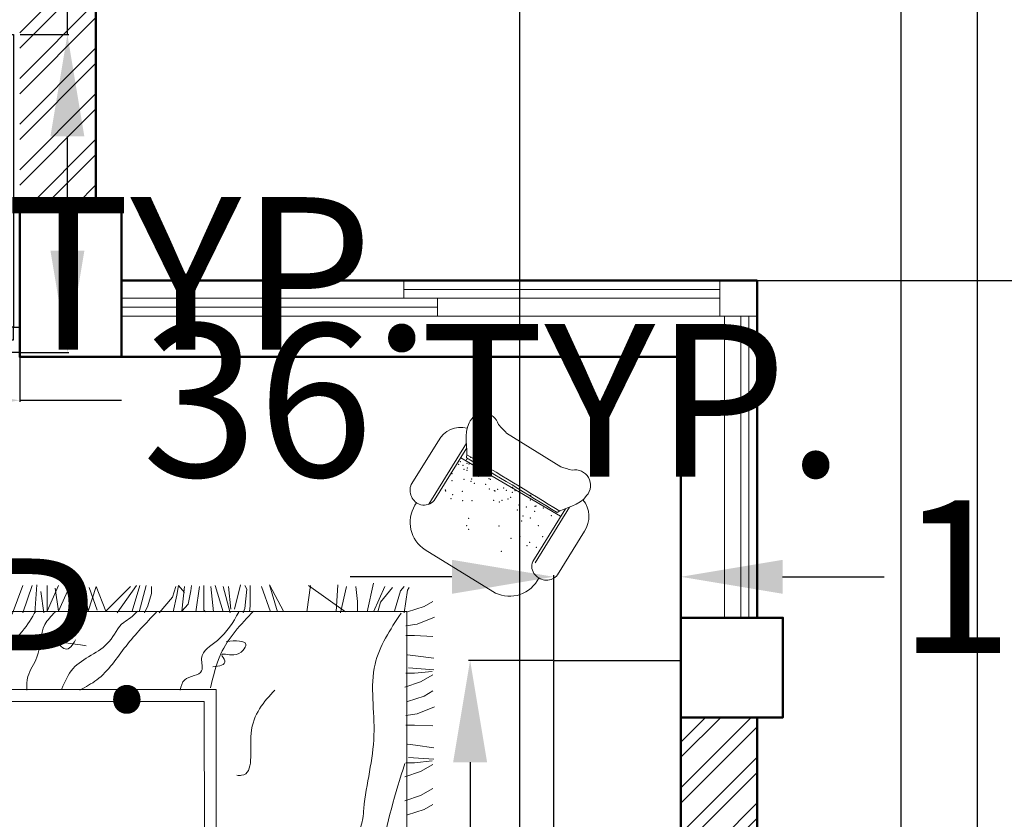
# Model space of a CAD drawing. Units: inches. Extents: x -90 to 536, y -553 to 299.
# Tile 25 of 27: x 294 to 410, y 80 to 174. Entities that reach past the tile are written whole.
import ezdxf

# ---------------------------------------------------------------- set-up
doc = ezdxf.new("R2010")
doc.units = ezdxf.units.IN
for name, color, linetype, lineweight in [('A-ANNO-DIMS', 2, 'Continuous', 18), ('A-COLS', 7, 'Continuous', 50), ('A-DOOR', 4, 'Continuous', 25), ('A-FLOR-CASE', 2, 'Continuous', 25), ('A-GLAZ', 4, 'Continuous', 18), ('A-WALL-PATT', 252, 'Continuous', 13), ('Furniture', 2, 'Continuous', 18), ('Outer Wall', 1, 'Continuous', 50)]:
    doc.layers.add(name, color=color, linetype=linetype, lineweight=lineweight)
doc.styles.get("Standard").update_dxf_attribs({"font": 'arial.ttf'})
doc.dimstyles.get("Standard").update_dxf_attribs({"dimtxt": 18, "dimasz": 12, "dimexe": 0.18, "dimexo": 0.0625, "dimgap": 0.09, "dimtad": 0, "dimtih": 1, "dimtoh": 1, "dimdec": 0, "dimzin": 0, "dimdsep": 46, "dimlunit": 3, "dimtxsty": 'Standard', "dimcen": 0.09, "dimadec": 0, "dimazin": 0, "dimtfac": 1, "dimtdec": 0, "dimtofl": 0, "dimtmove": 0, "dimatfit": 3, "dimfxl": 1, "dimtolj": 1, "dimtzin": 0, "dimarcsym": 0})

# ---------------------------------------------------------------- blocks, each defined once
blk = doc.blocks.new('A$C14440869')
for p, q in [((299.4, 786.8), (654.5, 786.8)), ((141.1, 259.3), (141.1, 621.8)), ((154.9, 258.1), (156.1, 601.9)), ((799, 258.1), (797.7, 601.9)), ((812.8, 224.7), (812.8, 621.8)), ((0, 267.1), (1, 551.8)), ((798, 537.4), (157.2, 552.6)), ((953.9, 267.1), (952.8, 551.8)), ((78.7, 198), (78.7, 179.8)), ((875.1, 196.3), (875.2, 179.8)), ((257.3, 0.1), (696.7, 0))]:
    blk.add_line(p, q)
for centre, radius, start, end in [((178, 741.7), 84.9, 46.4058, 190.9946), ((775.9, 741.7), 84.9, 349.0054, 133.5942), ((490.5, 1647.2), 881.3, 253.2515, 257.4746), ((463.3, 1647.2), 881.3, 282.5254, 286.7485), ((146, 557.8), 145.1, 108.7163, 182.3743), ((810.8, 559.8), 142.3, 356.766, 72.1434), ((234.9, -29958.2), 30532.1, 88.98134, 90.11086), ((164.3, -28909.7), 29469.6, 88.82111, 89.96326), ((79.9, 278.7), 80.7, 188.2473, 288.8842), ((90.3, 265.5), 65, 283.9696, 353.4821), ((871.6, 268.6), 73.4, 188.2144, 251.9677), ((869.8, 281.5), 85.3, 255.8372, 350.3327), ((257.8, 179.2), 179.2, 179.795, 269.795), ((696, 179.2), 179.2, 270.205, 0.205)]:
    blk.add_arc(centre, radius, start, end)
for points in [[(94.6, 725.5), (94.6, 660.2), (167.2, 599.5), (183.2, 559.8)], [(859.3, 725.5), (859.3, 660.2), (786.7, 599.5), (770.6, 553.6)]]:
    blk.add_open_spline(points, degree=3)
for p in [(358.4, 564.7), (467, 548.6), (656.1, 560.7), (752.6, 568.7), (201.4, 528.5), (261.8, 540.6), (294, 500.4), (302, 528.5), (306.1, 524.5), (346.3, 540.6), (346.3, 496.4), (446.9, 540.6), (446.9, 496.4), (454.9, 524.5), (487.1, 516.5), (507.2, 520.5), (531.4, 496.4), (595.7, 520.5), (603.8, 520.5), (647.8, 524.5), (651.8, 528.5), (656.1, 532.5), (656.1, 524.5), (659.9, 500.4), (688.3, 492.3), (692.1, 540.6), (696.3, 520.5), (700.3, 528.5), (732.5, 496.4), (736.6, 508.4), (740.6, 532.5), (748.6, 492.3), (752.4, 528.5), (764.7, 544.6), (764.7, 508.4), (788.9, 516.5), (788.9, 500.4), (233.6, 444.1), (294, 456.2), (334.2, 444.1), (378.5, 456.2), (386.5, 484.3), (454.9, 480.3), (479.1, 456.2), (487.1, 440.1), (539.4, 480.3), (543.4, 480.3), (571.6, 472.3), (603.8, 484.3), (659.9, 456.2), (680.2, 456.2), (684.2, 468.2), (720.2, 444.1), (181.3, 403.9), (326.2, 416), (519.3, 432.1), (692.3, 383.9), (772.5, 403.9), (792.9, 436.1), (181.3, 335.6), (225.6, 339.6), (290, 339.6), (418.7, 327.6), (619.9, 367.8), (663.9, 339.6), (728.3, 339.6), (772.5, 335.6), (776.8, 339.6), (229.6, 315.5), (326.2, 303.5), (583.7, 275.4), (724.3, 315.5), (551.5, 223.1), (571.6, 235.2), (334.2, 215.1)]:
    blk.add_point(p)
blk = doc.blocks.new('A$C2B723114')
for p, q in [((2.1776, 2.8509), (2.1776, 0.7454)), ((2.216, 2.8509), (2.216, 0.707)), ((2.4685, 1.4964), (2.4685, 0.0903)), ((2.4596, 1.3659), (2.552, 1.3324)), ((2.4645, 1.3318), (2.552, 1.3012)), ((2.4645, 1.2928), (2.5548, 1.2871)), ((2.4645, 1.2635), (2.5328, 1.2733)), ((2.4699, 1.2531), (2.552, 1.2163)), ((2.552, 1.2531), (2.4699, 1.2531)), ((2.5435, 1.2276), (2.4699, 1.2163)), ((2.4699, 1.2163), (2.5463, 1.1823)), ((2.5491, 1.1654), (2.467, 1.1597)), ((2.5463, 1.1455), (2.467, 1.1342)), ((2.5491, 1.1342), (2.4699, 1.1201)), ((2.4699, 1.1201), (2.5491, 1.0946)), ((2.5463, 1.1172), (2.4727, 1.0918)), ((2.5491, 1.0946), (2.4699, 1.0635)), ((2.4699, 1.0635), (2.5491, 0.9842)), ((2.4642, 1.0267), (2.552, 0.9644)), ((2.467, 0.9559), (2.552, 0.9333)), ((2.4699, 0.9785), (2.552, 0.9531)), ((2.4642, 0.9389), (2.4869, 0.9276)), ((2.4869, 0.9276), (2.5265, 0.9163)), ((2.5265, 0.9163), (2.5491, 0.9163)), ((2.4642, 0.8908), (2.5152, 0.8483)), ((2.467, 0.8455), (2.5208, 0.8342)), ((2.5152, 0.8483), (2.5491, 0.837)), ((2.5208, 0.8342), (2.552, 0.8285)), ((2.552, 0.8285), (2.5293, 0.8087)), ((2.4699, 0.8172), (2.4925, 0.7974)), ((2.5491, 0.8087), (2.4699, 0.8172)), ((2.4925, 0.7974), (2.535, 0.7889)), ((2.5491, 0.7606), (2.467, 0.7719)), ((2.535, 0.7889), (2.552, 0.7861)), ((2.1776, 0.7454), (0.7187, 0.7435)), ((2.4727, 0.7464), (2.467, 0.7408)), ((2.552, 0.7464), (2.4727, 0.7464)), ((2.216, 0.707), (0.6794, 0.7051)), ((2.467, 0.7153), (2.5491, 0.7238)), ((2.552, 0.7096), (2.467, 0.6842)), ((2.5491, 0.6842), (2.4642, 0.6615)), ((2.5491, 0.6672), (2.4755, 0.6587)), ((2.4755, 0.6474), (2.5548, 0.6276)), ((2.4642, 0.6191), (2.4784, 0.6134)), ((2.4784, 0.6134), (2.5406, 0.6077)), ((2.5406, 0.6077), (2.552, 0.6134)), ((2.467, 0.5993), (2.4869, 0.5964)), ((2.4869, 0.5964), (2.552, 0.5964)), ((2.467, 0.5313), (2.5491, 0.5596)), ((2.467, 0.5087), (2.5548, 0.5342)), ((2.5548, 0.5342), (2.4699, 0.4889)), ((2.467, 0.4133), (2.552, 0.4019)), ((2.467, 0.2879), (2.552, 0.4076)), ((2.467, 0.319), (2.5548, 0.3134)), ((2.4642, 0.3049), (2.5491, 0.2851)), ((2.4699, 0.2491), (2.501, 0.2491)), ((2.501, 0.2491), (2.5491, 0.2547)), ((2.467, 0.2179), (2.5605, 0.1981)), ((2.467, 0.1981), (2.5491, 0.1613)), ((2.467, 0.184), (2.4982, 0.1755)), ((2.4982, 0.1755), (2.5463, 0.1359)), ((2.4699, 0.1302), (2.535, 0.1104)), ((1.8568, 0.0962), (1.8738, 0.0453)), ((1.9342, 0.0962), (1.9512, 0.0453)), ((2.2236, 0.0962), (2.2406, 0.0453)), ((2.4642, 0.0991), (2.5378, 0.0877)), ((2.535, 0.1104), (2.5491, 0.0991)), ((2.4685, 0.0903), (0.4269, 0.0884)), ((1.8108, 0.0877), (1.8278, 0.034)), ((1.9795, 0.0934), (1.9795, 0.0651)), ((1.9795, 0.0651), (1.9852, 0.0085)), ((1.9965, 0.0849), (1.9908, 0.0028)), ((2.039, 0.0877), (2.0361, 0.0623)), ((2.1012, 0.0651), (2.0984, 0.0057)), ((2.1012, 0.0934), (2.1012, 0.0651)), ((2.1324, 0.0934), (2.138, 0.0566)), ((2.1777, 0.0877), (2.1946, 0.034)), ((2.2689, 0.0934), (2.2689, 0.0651)), ((2.2689, 0.0651), (2.2746, 0.0085)), ((2.2859, 0.0849), (2.2802, 0.0028)), ((2.3284, 0.0877), (2.3255, 0.0623)), ((2.3906, 0.0651), (2.3878, 0.0057)), ((2.3906, 0.0934), (2.3906, 0.0651)), ((2.4218, 0.0934), (2.4274, 0.0566)), ((2.467, 0.0877), (2.484, 0.034)), ((2.5378, 0.0877), (2.5463, 0.0821)), ((1.8278, 0.034), (1.8448, 0.0057)), ((1.8738, 0.0453), (1.8964, 0.0057)), ((1.9512, 0.0453), (1.9739, 0.0057)), ((2.0361, 0.0623), (2.0276, 0.0028)), ((2.138, 0.0566), (2.1607, 0)), ((2.1946, 0.034), (2.2116, 0.0057)), ((2.2406, 0.0453), (2.2632, 0.0057)), ((2.3255, 0.0623), (2.317, 0.0028)), ((2.4274, 0.0566), (2.4501, 0)), ((2.484, 0.034), (2.501, 0.0057))]:
    blk.add_line(p, q)
for points, knots in [([(2.2145, 1.4211), (2.233, 1.4246), (2.2636, 1.4303), (2.2761, 1.3837), (2.3429, 1.3967), (2.3949, 1.3342), (2.4474, 1.3031), (2.4698, 1.2898)], [0, 0, 0, 0, 61.886907, 102.717887, 145.699352, 284.082577, 386.765171, 386.765171, 386.765171, 386.765171]), ([(2.2145, 1.319), (2.2295, 1.319), (2.2678, 1.3192), (2.3288, 1.2705), (2.4143, 1.279), (2.4535, 1.2403), (2.4662, 1.2278)], [0, 0, 0, 0, 57.155505, 146.33427, 287.936209, 355.396728, 355.396728, 355.396728, 355.396728]), ([(2.3573, 1.127), (2.3656, 1.1759), (2.3758, 1.2352), (2.3371, 1.1853), (2.3602, 1.1713), (2.3768, 1.1612)], [0, 0, 0, 0, 107.853607, 130.728419, 189.220329, 189.220329, 189.220329, 189.220329]), ([(2.2182, 1.2059), (2.2419, 1.1958), (2.3116, 1.1659), (2.342, 1.0552), (2.4266, 1.0223), (2.4474, 0.9811), (2.462, 0.9684), (2.4698, 0.9616)], [0, 0, 0, 0, 97.73655, 287.59661, 389.176293, 423.403759, 463.679181, 463.679181, 463.679181, 463.679181]), ([(2.2145, 1.1476), (2.2246, 1.1286), (2.2575, 1.0666), (2.3612, 1.0009), (2.431, 0.9336), (2.4662, 0.8996)], [0, 0, 0, 0, 83.02987, 271.460712, 463.033803, 463.033803, 463.033803, 463.033803]), ([(2.2145, 0.823), (2.227, 0.8201), (2.261, 0.8121), (2.261, 0.7401), (2.3352, 0.7659), (2.379, 0.6836), (2.4336, 0.6521), (2.4662, 0.6334)], [0, 0, 0, 0, 46.747668, 127.438174, 179.649794, 280.561838, 429.605131, 429.605131, 429.605131, 429.605131]), ([(2.2218, 0.7246), (2.2595, 0.716), (2.3548, 0.6945), (2.4265, 0.6268), (2.4698, 0.586)], [0, 0, 0, 0, 148.665024, 375.555892, 375.555892, 375.555892, 375.555892]), ([(2.3719, 0.6737), (2.3738, 0.6431), (2.3772, 0.5878), (2.3146, 0.6382), (2.3401, 0.7015), (2.2971, 0.6649), (2.2923, 0.6965), (2.289, 0.7176)], [0, 0, 0, 0, 83.446591, 150.887818, 201.642461, 230.015204, 286.760644, 286.760644, 286.760644, 286.760644]), ([(2.2145, 0.5167), (2.1764, 0.5522), (2.1051, 0.6184), (1.9357, 0.5803), (1.9385, 0.6342), (1.9388, 0.6395)], [0, 0, 0, 0, 208.073343, 389.01094, 409.01094, 409.01094, 409.01094, 409.01094]), ([(2.4625, 0.1088), (2.4095, 0.1438), (2.2904, 0.2226), (2.0623, 0.1771), (1.9006, 0.2246), (1.7699, 0.2337), (1.6941, 0.2766), (1.5528, 0.2786), (1.4005, 0.2587), (1.2324, 0.3267), (1.059, 0.2939), (0.9218, 0.426), (0.7359, 0.3204), (0.5586, 0.2391), (0.4502, 0.3116), (0.427, 0.3272)], [0, 0, 0, 0, 239.874704, 538.942419, 850.40885, 893.390315, 1047.998294, 1176.505142, 1437.500972, 1637.333004, 1864.324391, 2089.058767, 2248.736533, 2637.953392, 2744.252142, 2744.252142, 2744.252142, 2744.252142]), ([(1.9771, 0.0962), (1.9286, 0.1117), (1.7864, 0.157), (1.5223, 0.1992), (1.2611, 0.141), (1.0527, 0.2023), (0.8859, 0.1885), (0.76, 0.3042), (0.6211, 0.292), (0.5187, 0.3203), (0.4572, 0.3456), (0.4282, 0.3575)], [0, 0, 0, 0, 198.710624, 582.73994, 1031.873213, 1206.082894, 1423.278209, 1655.952104, 1808.744089, 1945.69963, 2068.229211, 2068.229211, 2068.229211, 2068.229211])]:
    blk.add_open_spline(points, degree=3, knots=knots)
blk = doc.blocks.new('DOOR-36-A')
for points in [[(35.25, 37.5), (35.25, 3), (34.5, 3), (34.5, 37.5)], [(0, 0), (1.5, 0), (1.5, 1.5), (0.75, 1.5), (0.75, 3), (0, 3)], [(36, 0), (34.5, 0), (34.5, 1.5), (35.25, 1.5), (35.25, 3), (36, 3)]]:
    blk.add_lwpolyline(points, close=True)
blk.add_arc((37.64, 1.5), 36.14, 94.9791, 180)
blk = doc.blocks.new('COL-12X18')
blk.add_lwpolyline([(0, 18), (12, 18), (12, 0), (0, 0)], close=True)
blk = doc.blocks.new('COL-WINDOW-PIER')
blk.add_lwpolyline([(0, 11.76), (12.04, 11.76), (12.04, 0), (0, 0)], close=True)
blk = doc.blocks.new('TV-UNIT')
blk.add_lwpolyline([(15, 65.77), (15, 0), (0, 0), (0, 65.77)], close=True)
blk = doc.blocks.new('*D19')
at = {"layer": 'A-ANNO-DIMS', "color": 0, "lineweight": -2, "transparency": 16777216}
for p, q in [((299.76, 172.45), (299.76, 184.45)), ((299.76, 184.45), (311.76, 184.45)), ((294.19, 172.45), (299.94, 172.45)), ((299.76, 146.95), (299.76, 160.45)), ((294.19, 134.95), (299.94, 134.95))]:
    blk.add_line(p, q, dxfattribs=at)
at = {"layer": 'A-ANNO-DIMS', "color": 0, "transparency": 16777216}
for points in [[(297.76, 160.45), (301.76, 160.45), (299.76, 172.45)], [(297.76, 146.95), (301.76, 146.95), (299.76, 134.95)]]:
    blk.add_solid(points, dxfattribs=at)
at = {"layer": 'Defpoints', "color": 0, "transparency": 16777216}
for p in [(294.13, 172.45), (299.76, 172.45), (294.13, 134.95)]:
    blk.add_point(p, dxfattribs=at)
at = {"layer": 'A-ANNO-DIMS', "color": 0, "transparency": 16777216, "insert": (408.3, 184.45), "char_height": 18, "attachment_point": 5}
blk.add_mtext('\\A1;DOOR A 38 TYP.', dxfattribs=at)
blk = doc.blocks.new('*D20')
at = {"layer": 'A-ANNO-DIMS', "color": 0, "lineweight": -2, "transparency": 16777216}
for p, q in [((258.13, 134.88), (258.13, 129.14)), ((294.13, 134.88), (294.13, 129.14)), ((270.13, 129.32), (282.13, 129.32)), ((294.13, 129.32), (306.13, 129.32))]:
    blk.add_line(p, q, dxfattribs=at)
at = {"layer": 'A-ANNO-DIMS', "color": 0, "transparency": 16777216}
for points in [[(270.13, 131.32), (270.13, 127.32), (258.13, 129.32)], [(282.13, 131.32), (282.13, 127.32), (294.13, 129.32)]]:
    blk.add_solid(points, dxfattribs=at)
at = {"layer": 'Defpoints', "color": 0, "transparency": 16777216}
for p in [(258.13, 134.95), (294.13, 134.95), (294.13, 129.32)]:
    blk.add_point(p, dxfattribs=at)
at = {"layer": 'A-ANNO-DIMS', "color": 0, "transparency": 16777216, "insert": (350.02, 129.32), "char_height": 18, "attachment_point": 5}
blk.add_mtext('\\A1;36 TYP.', dxfattribs=at)
blk = doc.blocks.new('*D25')
at = {"layer": 'A-ANNO-DIMS', "color": 0, "lineweight": -2, "transparency": 16777216}
for p, q in [((228.95, 178.94), (228.95, 190.94)), ((228.95, 190.94), (240.95, 190.94)), ((226.49, 166.94), (229.13, 166.94)), ((226.49, 150.15), (229.13, 150.15)), ((228.95, 138.15), (228.95, 126.15))]:
    blk.add_line(p, q, dxfattribs=at)
at = {"layer": 'A-ANNO-DIMS', "color": 0, "transparency": 16777216}
for points in [[(226.95, 178.94), (230.95, 178.94), (228.95, 166.94)], [(226.95, 138.15), (230.95, 138.15), (228.95, 150.15)]]:
    blk.add_solid(points, dxfattribs=at)
at = {"layer": 'Defpoints', "color": 0, "transparency": 16777216}
for p in [(226.43, 166.94), (228.95, 166.94), (226.43, 150.15)]:
    blk.add_point(p, dxfattribs=at)
at = {"layer": 'A-ANNO-DIMS', "color": 0, "transparency": 16777216, "insert": (325.67, 190.94), "char_height": 18, "attachment_point": 5}
blk.add_mtext('\\A1;BASIN 17 TYP.', dxfattribs=at)
blk = doc.blocks.new('*D29')
at = {"layer": 'A-ANNO-DIMS', "color": 0, "lineweight": -2, "transparency": 16777216}
for p, q in [((357.07, 98.65), (347.09, 98.65)), ((347.27, 86.65), (347.27, 75.05)), ((347.27, 44.88), (347.27, 56.48)), ((357.07, 32.88), (347.09, 32.88))]:
    blk.add_line(p, q, dxfattribs=at)
at = {"layer": 'A-ANNO-DIMS', "color": 0, "transparency": 16777216}
for points in [[(345.27, 86.65), (349.27, 86.65), (347.27, 98.65)], [(345.27, 44.88), (349.27, 44.88), (347.27, 32.88)]]:
    blk.add_solid(points, dxfattribs=at)
at = {"layer": 'Defpoints', "color": 0, "transparency": 16777216}
for p in [(347.27, 98.65), (357.13, 98.65), (357.13, 32.88)]:
    blk.add_point(p, dxfattribs=at)
at = {"layer": 'A-ANNO-DIMS', "color": 0, "transparency": 16777216, "insert": (347.27, 65.76), "char_height": 18, "attachment_point": 5}
blk.add_mtext('\\A1;TV UNIT 66 TYP.', dxfattribs=at)
blk = doc.blocks.new('*D30')
at = {"layer": 'A-ANNO-DIMS', "color": 0, "lineweight": -2, "transparency": 16777216}
for p, q in [((345.13, 108.51), (333.13, 108.51)), ((357.13, 98.71), (357.13, 108.69)), ((372.13, 98.71), (372.13, 108.69)), ((384.13, 108.51), (396.13, 108.51))]:
    blk.add_line(p, q, dxfattribs=at)
at = {"layer": 'A-ANNO-DIMS', "color": 0, "transparency": 16777216}
for points in [[(345.13, 110.51), (345.13, 106.51), (357.13, 108.51)], [(384.13, 110.51), (384.13, 106.51), (372.13, 108.51)]]:
    blk.add_solid(points, dxfattribs=at)
at = {"layer": 'Defpoints', "color": 0, "transparency": 16777216}
for p in [(372.13, 108.51), (357.13, 98.65), (372.13, 98.65)]:
    blk.add_point(p, dxfattribs=at)
at = {"layer": 'A-ANNO-DIMS', "color": 0, "transparency": 16777216, "insert": (439.18, 108.51), "char_height": 18, "attachment_point": 5}
blk.add_mtext('\\A1;15 TYP.', dxfattribs=at)
blk = doc.blocks.new('*D33')
at = {"layer": 'A-ANNO-DIMS', "color": 0, "lineweight": -2, "transparency": 16777216}
for p, q in [((173.76, 108.4), (189.77, 108.4)), ((189.59, 96.4), (189.59, 64.83)), ((189.59, 14.45), (189.59, 46.02)), ((173.76, 2.45), (189.77, 2.45))]:
    blk.add_line(p, q, dxfattribs=at)
at = {"layer": 'A-ANNO-DIMS', "color": 0, "transparency": 16777216}
for points in [[(187.59, 96.4), (191.59, 96.4), (189.59, 108.4)], [(187.59, 14.45), (191.59, 14.45), (189.59, 2.45)]]:
    blk.add_solid(points, dxfattribs=at)
at = {"layer": 'Defpoints', "color": 0, "transparency": 16777216}
for p in [(173.7, 108.4), (173.7, 2.45), (189.59, 2.45)]:
    blk.add_point(p, dxfattribs=at)
at = {"layer": 'A-ANNO-DIMS', "color": 0, "transparency": 16777216, "insert": (189.59, 55.42), "char_height": 18, "attachment_point": 5}
blk.add_mtext('\\A1;BED GROUP 106 TYP.', dxfattribs=at)
blk = doc.blocks.new('*D39')
at = {"layer": 'A-ANNO-DIMS', "color": 0, "lineweight": -2, "transparency": 16777216}
for p, q in [((209.07, 134.45), (199.12, 134.45)), ((199.3, 122.45), (199.3, 111.07)), ((199.3, 80.89), (199.3, 92.26)), ((209.07, 68.89), (199.12, 68.89))]:
    blk.add_line(p, q, dxfattribs=at)
at = {"layer": 'A-ANNO-DIMS', "color": 0, "transparency": 16777216}
for points in [[(197.3, 122.45), (201.3, 122.45), (199.3, 134.45)], [(197.3, 80.89), (201.3, 80.89), (199.3, 68.89)]]:
    blk.add_solid(points, dxfattribs=at)
at = {"layer": 'Defpoints', "color": 0, "transparency": 16777216}
for p in [(199.3, 134.45), (209.13, 134.45), (209.13, 68.89)]:
    blk.add_point(p, dxfattribs=at)
at = {"layer": 'A-ANNO-DIMS', "color": 0, "transparency": 16777216, "insert": (199.3, 101.67), "char_height": 18, "attachment_point": 5}
blk.add_mtext('\\A1;WARDROBE 66 TYP.', dxfattribs=at)
blk = doc.blocks.new('*D40')
at = {"layer": 'A-ANNO-DIMS', "color": 0, "lineweight": -2, "transparency": 16777216}
for p, q in [((197.13, 144.28), (185.13, 144.28)), ((209.13, 134.51), (209.13, 144.46)), ((233.13, 134.51), (233.13, 144.46)), ((245.13, 144.28), (257.13, 144.28))]:
    blk.add_line(p, q, dxfattribs=at)
at = {"layer": 'A-ANNO-DIMS', "color": 0, "transparency": 16777216}
for points in [[(197.13, 146.28), (197.13, 142.28), (209.13, 144.28)], [(245.13, 146.28), (245.13, 142.28), (233.13, 144.28)]]:
    blk.add_solid(points, dxfattribs=at)
at = {"layer": 'Defpoints', "color": 0, "transparency": 16777216}
for p in [(233.13, 144.28), (209.13, 134.45), (233.13, 134.45)]:
    blk.add_point(p, dxfattribs=at)
at = {"layer": 'A-ANNO-DIMS', "color": 0, "transparency": 16777216, "insert": (301.18, 144.28), "char_height": 18, "attachment_point": 5}
blk.add_mtext('\\A1;24 TYP.', dxfattribs=at)
blk = doc.blocks.new('*D53')
at = {"layer": 'A-ANNO-DIMS', "color": 0, "lineweight": -2, "transparency": 16777216}
for p, q in [((35.09, 103.75), (35.09, 287.38)), ((47.09, 287.2), (183.7, 287.2)), ((395.13, 287.2), (258.52, 287.2)), ((407.13, -63.49), (407.13, 287.38))]:
    blk.add_line(p, q, dxfattribs=at)
at = {"layer": 'A-ANNO-DIMS', "color": 0, "transparency": 16777216}
for points in [[(47.09, 289.2), (47.09, 285.2), (35.09, 287.2)], [(395.13, 289.2), (395.13, 285.2), (407.13, 287.2)]]:
    blk.add_solid(points, dxfattribs=at)
at = {"layer": 'Defpoints', "color": 0, "transparency": 16777216}
for p in [(407.13, 287.2), (35.09, 103.69), (407.13, -63.55)]:
    blk.add_point(p, dxfattribs=at)
at = {"layer": 'A-ANNO-DIMS', "color": 0, "transparency": 16777216, "insert": (221.11, 287.2), "char_height": 18, "attachment_point": 5}
blk.add_mtext('\\A1;372.04', dxfattribs=at)
blk = doc.blocks.new('*D58')
at = {"layer": 'A-ANNO-DIMS', "color": 0, "lineweight": -2, "transparency": 16777216}
for p, q in [((290.13, -71.49), (290.13, 287.38)), ((302.13, 287.2), (308.6, 287.2)), ((341.13, 287.2), (334.66, 287.2)), ((353.13, -71.49), (353.13, 287.38))]:
    blk.add_line(p, q, dxfattribs=at)
at = {"layer": 'A-ANNO-DIMS', "color": 0, "transparency": 16777216}
for points in [[(302.13, 289.2), (302.13, 285.2), (290.13, 287.2)], [(341.13, 289.2), (341.13, 285.2), (353.13, 287.2)]]:
    blk.add_solid(points, dxfattribs=at)
at = {"layer": 'Defpoints', "color": 0, "transparency": 16777216}
for p in [(353.13, 287.2), (290.13, -71.55), (353.13, -71.55)]:
    blk.add_point(p, dxfattribs=at)
at = {"layer": 'A-ANNO-DIMS', "color": 0, "transparency": 16777216, "insert": (321.63, 287.2), "char_height": 18, "attachment_point": 5}
blk.add_mtext('\\A1;63', dxfattribs=at)
blk = doc.blocks.new('*D59')
at = {"layer": 'A-ANNO-DIMS', "color": 0, "lineweight": -2, "transparency": 16777216}
for p, q in [((341.13174, 287.201217), (329.13174, 287.201217)), ((353.13174, -71.491283), (353.13174, 287.381217)), ((398.13174, -71.491283), (398.13174, 287.381217)), ((410.13174, 287.201217), (422.13174, 287.201217))]:
    blk.add_line(p, q, dxfattribs=at)
at = {"layer": 'A-ANNO-DIMS', "color": 0, "transparency": 16777216}
for points in [[(341.13174, 289.201217), (341.13174, 285.201217), (353.13174, 287.201217)], [(410.13174, 289.201217), (410.13174, 285.201217), (398.13174, 287.201217)]]:
    blk.add_solid(points, dxfattribs=at)
at = {"layer": 'Defpoints', "color": 0, "transparency": 16777216}
for p in [(398.13174, 287.201217), (353.13174, -71.553783), (398.13174, -71.553783)]:
    blk.add_point(p, dxfattribs=at)
at = {"layer": 'A-ANNO-DIMS', "color": 0, "transparency": 16777216, "insert": (375.63174, 287.201217), "char_height": 18, "attachment_point": 5}
blk.add_mtext('\\A1;45', dxfattribs=at)
blk = doc.blocks.new('*D66')
at = {"layer": 'A-ANNO-DIMS', "color": 0, "lineweight": -2, "transparency": 16777216}
for p, q in [((303.19, 249.45), (445.07, 249.45)), ((444.89, 237.45), (444.89, 205.73)), ((444.89, 155.45), (444.89, 187.17)), ((381.19, 143.45), (445.07, 143.45))]:
    blk.add_line(p, q, dxfattribs=at)
at = {"layer": 'A-ANNO-DIMS', "color": 0, "transparency": 16777216}
for points in [[(442.89, 237.45), (446.89, 237.45), (444.89, 249.45)], [(442.89, 155.45), (446.89, 155.45), (444.89, 143.45)]]:
    blk.add_solid(points, dxfattribs=at)
at = {"layer": 'Defpoints', "color": 0, "transparency": 16777216}
for p in [(303.13, 249.45), (444.89, 249.45), (381.13, 143.45)]:
    blk.add_point(p, dxfattribs=at)
at = {"layer": 'A-ANNO-DIMS', "color": 0, "transparency": 16777216, "insert": (444.89, 196.45), "char_height": 18, "attachment_point": 5}
blk.add_mtext('\\A1;106', dxfattribs=at)

msp = doc.modelspace()

# ---------------------------------------------------------------- hatches: boundary and pattern name
at = {"layer": 'A-WALL-PATT'}
h = msp.add_hatch(dxfattribs=at)
h.set_pattern_fill('ANSI32', color=256, scale=0.4)
h.set_pattern_definition([(45, (-88.8105, -603.6155), (-2.694077, 2.694077), []), (45, (-87.0145, -603.6155), (-2.694077, 2.694077), [])])
h.paths.add_polyline_path([(285.1317, 246.4462), (131.1317, 246.4462), (131.1317, 237.4462), (285.1317, 237.4462)])
h.paths.add_polyline_path([(122.1317, 237.4462), (113.1317, 237.4462), (113.1317, 152.4462), (122.1317, 152.4462), (122.1317, 166.4704)])
h.paths.add_polyline_path([(303.1317, 237.4462), (294.1317, 237.4462), (294.1317, 152.4462), (303.1317, 152.4462)])
h.paths.add_polyline_path([(47.1317, 91.9277), (38.1317, 91.9277), (38.1317, -6.5538), (77.1317, -6.5538), (77.1317, 2.4462), (70.5655, 2.4462), (47.1317, 2.4462)])
h.paths.add_polyline_path([(83.052, -61.5538), (47.1317, -61.5538), (47.1317, -24.5538), (38.1317, -24.5538), (38.1317, -70.5538), (74.052, -70.5538), (74.052, -223.5538), (38.1317, -223.5538), (38.1317, -503.5538), (92.1317, -503.5538), (92.1317, -437.5538), (191.1317, -437.5538), (191.1317, -428.5538), (83.1317, -428.5538), (83.1317, -494.5538), (47.1317, -494.5538), (47.1317, -232.5538), (83.052, -232.5538), (83.052, -70.5538)])
h.paths.add_polyline_path([(407.1317, -63.5538), (381.1317, -63.5538), (381.1317, 91.9277), (372.1317, 91.9277), (372.1317, 32.8805), (372.1317, -63.5538), (306.5745, -63.5538), (237.1317, -63.5538), (237.1317, -38.5538), (233.1317, -38.5538), (233.1317, -71.5538), (398.1317, -71.5538), (398.1317, -152.5538), (233.1317, -152.5538), (233.1317, -161.5538), (398.1317, -161.5538), (398.1317, -368.5538), (233.1317, -368.5538), (233.1317, -377.5538), (407.1317, -377.5538), (407.1317, -161.5538)])
h.paths.add_polyline_path([(261.1317, -422.5538), (252.1317, -422.5538), (252.1317, -428.5538), (233.1317, -428.5538), (233.1317, -437.5538), (261.1317, -437.5538)])
h.paths.add_polyline_path([(191.1317, -368.5538), (180.1317, -368.5538), (180.1317, -335.5538), (131.5919, -335.5538), (131.5919, -344.5538), (171.1317, -344.5538), (171.1317, -392.5538), (180.1317, -392.5538), (180.1317, -377.5538), (191.1317, -377.5538)], flags=17)
h.paths.add_polyline_path([(180.1317, -223.5538), (152.1317, -223.5538), (152.1317, -227.5538), (176.1317, -227.5538), (176.1317, -335.5538), (180.1317, -335.5538)], flags=17)
h.paths.add_polyline_path([(131.5919, -335.5538), (83.1317, -335.5538), (83.1317, -339.5538), (83.1317, -392.5538), (87.1317, -392.5538), (87.1317, -339.5538), (131.5919, -339.5538)], flags=17)
h.paths.add_polyline_path([(197.1317, 2.4462), (77.1317, 2.4462), (77.1317, -1.5538), (113.1317, -1.5538), (113.1317, -71.5538), (181.1317, -71.5538), (181.1317, -67.5538), (117.1317, -67.5538), (117.1317, -1.5538), (177.1317, -1.5538), (177.1317, -37.5538), (181.1317, -37.5538), (181.1317, -1.5538), (197.1317, -1.5538)])
h.paths.add_polyline_path([(173.1317, 138.4462), (122.1317, 138.4462), (122.1317, 134.4462), (173.1317, 134.4462)])
h.paths.add_polyline_path([(213.1317, 237.4462), (209.1317, 237.4462), (209.1317, 134.4462), (233.1317, 134.4462), (233.1317, 68.8889), (233.1317, -2.5538), (237.1317, -2.5538), (237.1317, 134.4462), (258.1317, 134.4462), (258.1317, 138.4462), (213.1317, 138.4462)])

# ---------------------------------------------------------------- linework, layer by layer
at = {"layer": 'A-GLAZ'}
for p, q in [((339.4315, 142.4), (376.7312, 142.4)), ((306.1317, 140.3075), (343.4315, 140.3075)), ((341.4315, 139.2612), (376.7312, 139.2612)), ((377.2863, 139.2612), (377.2863, 103.6916)), ((380.1704, 139.2612), (380.1704, 103.6916))]:
    msp.add_line(p, q, dxfattribs=at)
for points in [[(376.7312, 143.4462), (339.4315, 143.4462), (339.4315, 141.3537), (376.7312, 141.3537)], [(381.1317, 143.4462), (376.7312, 143.4462), (376.7312, 139.2612), (381.1317, 139.2612)], [(306.1317, 139.2612), (343.4315, 139.2612), (343.4315, 141.3537), (306.1317, 141.3537)], [(381.1317, 139.2612), (379.209, 139.2612), (379.209, 103.6916), (381.1317, 103.6916)]]:
    msp.add_lwpolyline(points, close=True, dxfattribs=at)
at = {"layer": 'Outer Wall'}
for p, q in [((303.1317, 246.4462), (303.1317, 152.4462)), ((381.1317, 143.4462), (306.1317, 143.4462)), ((381.1317, 143.4462), (381.1317, 103.6916)), ((372.1317, 134.4462), (306.1317, 134.4462)), ((372.1317, 134.4462), (372.1317, -63.5538)), ((381.1317, 91.9277), (381.1317, -63.5538))]:
    msp.add_line(p, q, dxfattribs=at)

# ---------------------------------------------------------------- block references
at = {"layer": 'A-COLS'}
for name, p in [('COL-12X18', (294.1317, 134.4462)), ('COL-WINDOW-PIER', (372.1317, 91.9277))]:
    msp.add_blockref(name, p, dxfattribs=at)
at = {"layer": 'A-DOOR'}
msp.add_blockref('DOOR-36-A', (258.1317, 134.9462), dxfattribs=at)
at = {"layer": 'A-FLOR-CASE'}
msp.add_blockref('TV-UNIT', (357.1317, 32.8805), dxfattribs=at)
at = {"layer": 'Furniture'}
for name, p, xscale, yscale, zscale, rotation in [('A$C14440869', (354.5892, 103.8956), -0.0212813664299499, 0.0212813664299499, 0.0212813664299499, 328.2432984708461), ('A$C2B723114', (343.0864, 14.3799), 36.47664764473289, 36.47664764473289, 36.47664764473289, 89.99999999999999)]:
    msp.add_blockref(name, p, dxfattribs=dict(at, xscale=xscale, yscale=yscale, zscale=zscale, rotation=rotation))

# ---------------------------------------------------------------- dimensions: what is measured, and where the dimension line sits
at = {"layer": 'A-ANNO-DIMS'}
for base, p1, p2, override, picture, middle in [((407.1317, 287.2012), (35.0873, 103.6916), (407.1317, -63.5538), {"dimdec": 2, "dimlfac": 1, "dimrnd": 0, "dimzin": 0, "dimdsep": 46, "dimlunit": 2}, '*D53', (221.1095, 287.2012)), ((353.1317, 287.2012), (290.1317, -71.5538), (353.1317, -71.5538), {"dimdec": 0, "dimlfac": 1, "dimrnd": 0, "dimzin": 0, "dimdsep": 46, "dimlunit": 2}, '*D58', (321.6317, 287.2012)), ((398.1317, 287.2012), (353.1317, -71.5538), (398.1317, -71.5538), {"dimdec": 0, "dimlfac": 1, "dimrnd": 0, "dimzin": 0, "dimdsep": 46, "dimlunit": 2}, '*D59', (375.6317, 287.2012))]:
    dim = msp.add_linear_dim(base=base, p1=p1, p2=p2, dimstyle='Standard', override=override, dxfattribs=at)
    dim.commit()
    dim.dimension.update_dxf_attribs({"geometry": picture, "text_midpoint": middle})
dim = msp.add_linear_dim(base=(444.8867, 249.4462), p1=(381.1317, 143.4462), p2=(303.1317, 249.4462), angle=90, dimstyle='Standard', override={"dimdec": 0, "dimlfac": 1, "dimrnd": 0, "dimzin": 0, "dimdsep": 46, "dimlunit": 2}, dxfattribs=at)
dim.commit()
dim.dimension.update_dxf_attribs({"geometry": '*D66', "text_midpoint": (444.8867, 196.4462)})
for base, p1, p2, angle, text, picture, middle in [((299.7567404714, 172.4462174295), (294.1317404714, 134.9462174295), (294.1317404714, 172.4462174295), 90, 'DOOR A <> TYP.', '*D19', (408.2989914946, 184.4462174295)), ((228.949, 166.9352), (226.4312, 150.1495), (226.4312, 166.9352), 90, 'BASIN <> TYP.', '*D25', (325.6734, 190.9352)), ((199.2981, 134.4462), (209.1317, 68.8889), (209.1317, 134.4462), 90, 'WARDROBE <> TYP.', '*D39', (199.2981, 101.6676)), ((347.2664, 98.6495), (357.1317, 32.8805), (357.1317, 98.6495), 90, 'TV UNIT <> TYP.', '*D29', (347.2664, 65.765)), ((189.5912, 2.4462), (173.698, 108.4009), (173.698, 2.4462), 270, 'BED GROUP <> TYP.', '*D33', (189.5912, 55.4235))]:
    dim = msp.add_linear_dim(base=base, p1=p1, p2=p2, angle=angle, text=text, dimstyle='Standard', override={"dimdec": 0, "dimlfac": 1, "dimrnd": 0, "dimzin": 0, "dimdsep": 46, "dimlunit": 2}, dxfattribs=at)
    dim.commit()
    dim.dimension.update_dxf_attribs({"geometry": picture, "text_midpoint": middle})
for base, p1, p2, picture, middle in [((233.1317, 144.2798), (209.1317, 134.4462), (233.1317, 134.4462), '*D40', (301.1842, 144.2798)), ((294.1317, 129.3212), (258.1317, 134.9462), (294.1317, 134.9462), '*D20', (350.0246, 129.3212)), ((372.1317, 108.5148), (357.1317, 98.6495), (372.1317, 98.6495), '*D30', (439.1835, 108.5148))]:
    dim = msp.add_linear_dim(base=base, p1=p1, p2=p2, text='<> TYP.', dimstyle='Standard', override={"dimdec": 0, "dimlfac": 1, "dimrnd": 0, "dimzin": 0, "dimdsep": 46, "dimlunit": 2}, dxfattribs=at)
    dim.commit()
    dim.dimension.update_dxf_attribs({"geometry": picture, "text_midpoint": middle})

doc.saveas('drawing.dxf')
